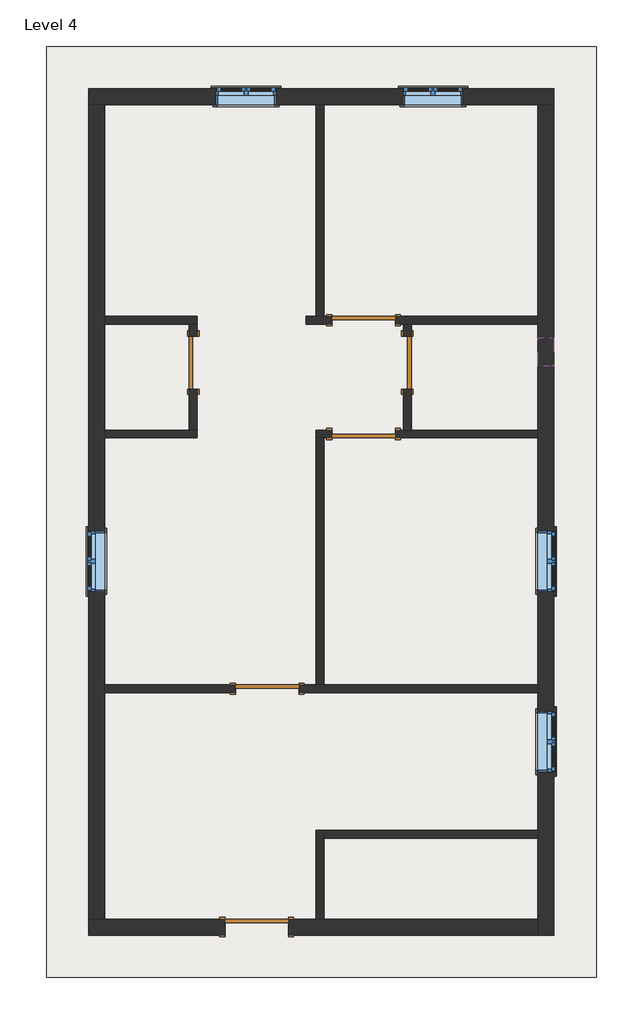
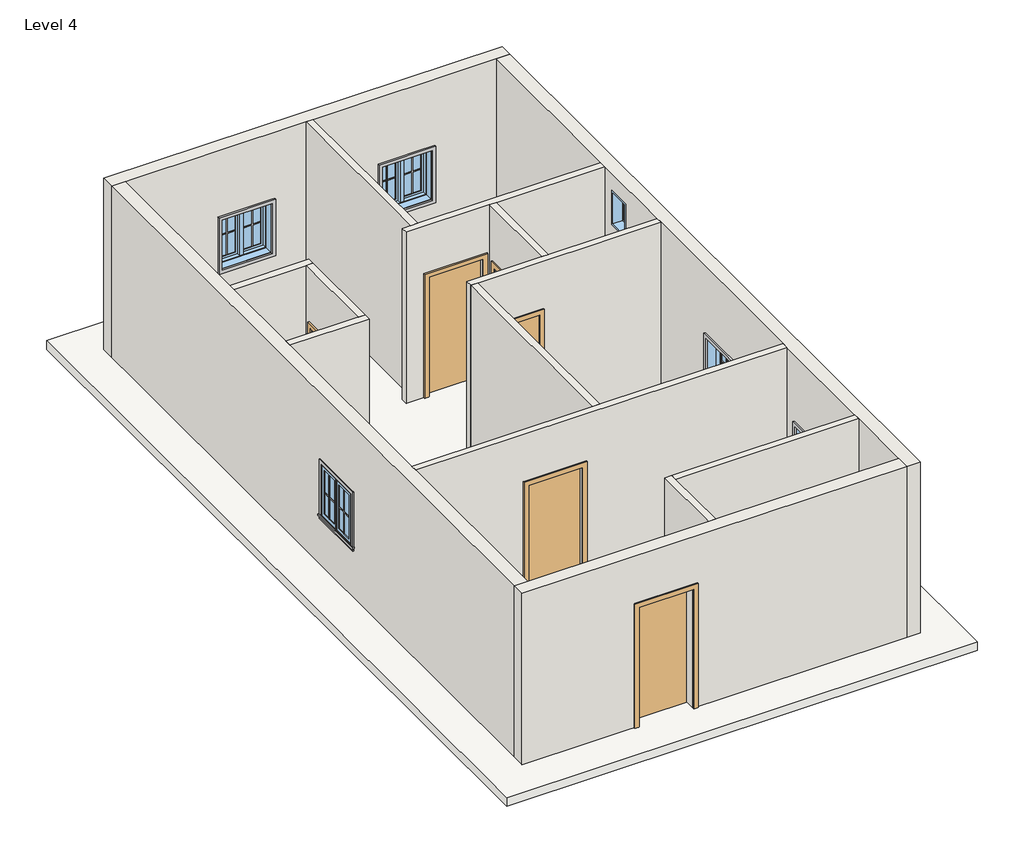
# One storey, incomplete: 20 proxies, 15 walls, 6 doors, 6 windows, 1 roof.
"""IFC4 building model written with IfcOpenShell, lengths in millimetres."""

from ifc_helpers import new_model, si_unit, frame, origin, place, context, project, spatial, polyline, outline, extrude, faceted_brep, transform, mapped, element, save
from components import muntin_pattern_2x2_muntin_pattern_2x2_b3fe6957, muntin_pattern_2x2_muntin_pattern_2x2_3e0ecaf2, trim_window_exterior_flat_with_sill_41619996, trim_window_interior_flat_picture_frame_51c85655, door_f2b275c1, door_d8f5dbb5, door_305aa2a5, door_e5f9f3c4, door_a90ba1ad, window_aa618e30, window_339605e1

model = new_model("IFC4")

# Units and contexts
model_context = context("Model", 3, world=origin())
ifc_project = project(units=[si_unit("LENGTHUNIT", "METRE", prefix="MILLI")], contexts=[model_context])

# Site, building, storey
site = spatial("IfcSite", under=ifc_project)
building = spatial("IfcBuilding", under=site)
storey = spatial("IfcBuildingStorey", under=building, Name="Level 4", Elevation=6400.8)

# Proxies
placement = place(None, origin())
muntin_pattern_2x2_muntin_pattern_2x2_shape = muntin_pattern_2x2_muntin_pattern_2x2_b3fe6957(model_context)
element("IfcBuildingElementProxy", 1, Name="Muntin Pattern_2x2 : Muntin Pattern_2x2", ObjectType="Muntin Pattern_2x2 : Muntin Pattern_2x2", at=placement, inside=storey, context=model_context, shape_type="MappedRepresentation", body=[
    mapped(muntin_pattern_2x2_muntin_pattern_2x2_shape, transform((-2560.703247, 6624.6685985, 7385.05), x_axis=(1.0, 0.0, 0.0), y_axis=(0.0, 1.0, 0.0), z_axis=(0.0, 0.0, 1.0))),
])
element("IfcBuildingElementProxy", 2, Name="Muntin Pattern_2x2 : Muntin Pattern_2x2", ObjectType="Muntin Pattern_2x2 : Muntin Pattern_2x2", at=placement, inside=storey, context=model_context, shape_type="MappedRepresentation", body=[
    mapped(muntin_pattern_2x2_muntin_pattern_2x2_shape, transform((134.871753, 6624.6685985, 7385.05), x_axis=(1.0, 0.0, 0.0), y_axis=(0.0, 1.0, 0.0), z_axis=(0.0, 0.0, 1.0))),
])
element("IfcBuildingElementProxy", 3, Name="Muntin Pattern_2x2 : Muntin Pattern_2x2", ObjectType="Muntin Pattern_2x2 : Muntin Pattern_2x2", at=placement, inside=storey, context=model_context, shape_type="MappedRepresentation", body=[
    mapped(muntin_pattern_2x2_muntin_pattern_2x2_shape, transform((2082.734253, 41.3060985, 7385.05), x_axis=(0.0, -1.0, 0.0), y_axis=(1.0, 0.0, 0.0), z_axis=(0.0, 0.0, 1.0))),
])
element("IfcBuildingElementProxy", 4, Name="Muntin Pattern_2x2 : Muntin Pattern_2x2", ObjectType="Muntin Pattern_2x2 : Muntin Pattern_2x2", at=placement, inside=storey, context=model_context, shape_type="MappedRepresentation", body=[
    mapped(muntin_pattern_2x2_muntin_pattern_2x2_shape, transform((-4603.815747, -387.3189015, 7385.05), x_axis=(0.0, 1.0, 0.0), y_axis=(-1.0, 0.0, 0.0), z_axis=(0.0, 0.0, 1.0))),
])
element("IfcBuildingElementProxy", 5, Name="Muntin Pattern_2x2 : Muntin Pattern_2x2", ObjectType="Muntin Pattern_2x2 : Muntin Pattern_2x2", at=placement, inside=storey, context=model_context, shape_type="MappedRepresentation", body=[
    mapped(muntin_pattern_2x2_muntin_pattern_2x2_shape, transform((2082.734253, -2555.8439015, 7385.05), x_axis=(0.0, -1.0, 0.0), y_axis=(1.0, 0.0, 0.0), z_axis=(0.0, 0.0, 1.0))),
])
muntin_pattern_2x2_muntin_pattern_2x2_2_shape = muntin_pattern_2x2_muntin_pattern_2x2_3e0ecaf2(model_context)
element("IfcBuildingElementProxy", 6, Name="Muntin Pattern_2x2 : Muntin Pattern_2x2", ObjectType="Muntin Pattern_2x2 : Muntin Pattern_2x2", at=placement, inside=storey, context=model_context, shape_type="MappedRepresentation", body=[
    mapped(muntin_pattern_2x2_muntin_pattern_2x2_2_shape, transform((-2132.078247, 6624.6685985, 7385.05), x_axis=(-1.0, 0.0, 0.0), y_axis=(0.0, -1.0, 0.0), z_axis=(0.0, 0.0, 1.0))),
])
element("IfcBuildingElementProxy", 7, Name="Muntin Pattern_2x2 : Muntin Pattern_2x2", ObjectType="Muntin Pattern_2x2 : Muntin Pattern_2x2", at=placement, inside=storey, context=model_context, shape_type="MappedRepresentation", body=[
    mapped(muntin_pattern_2x2_muntin_pattern_2x2_2_shape, transform((563.496753, 6624.6685985, 7385.05), x_axis=(-1.0, 0.0, 0.0), y_axis=(0.0, -1.0, 0.0), z_axis=(0.0, 0.0, 1.0))),
])
element("IfcBuildingElementProxy", 8, Name="Muntin Pattern_2x2 : Muntin Pattern_2x2", ObjectType="Muntin Pattern_2x2 : Muntin Pattern_2x2", at=placement, inside=storey, context=model_context, shape_type="MappedRepresentation", body=[
    mapped(muntin_pattern_2x2_muntin_pattern_2x2_2_shape, transform((2082.734253, -387.3189015, 7385.05), x_axis=(0.0, 1.0, 0.0), y_axis=(-1.0, 0.0, 0.0), z_axis=(0.0, 0.0, 1.0))),
])
element("IfcBuildingElementProxy", 9, Name="Muntin Pattern_2x2 : Muntin Pattern_2x2", ObjectType="Muntin Pattern_2x2 : Muntin Pattern_2x2", at=placement, inside=storey, context=model_context, shape_type="MappedRepresentation", body=[
    mapped(muntin_pattern_2x2_muntin_pattern_2x2_2_shape, transform((-4603.815747, 41.3060985, 7385.05), x_axis=(0.0, -1.0, 0.0), y_axis=(1.0, 0.0, 0.0), z_axis=(0.0, 0.0, 1.0))),
])
element("IfcBuildingElementProxy", 10, Name="Muntin Pattern_2x2 : Muntin Pattern_2x2", ObjectType="Muntin Pattern_2x2 : Muntin Pattern_2x2", at=placement, inside=storey, context=model_context, shape_type="MappedRepresentation", body=[
    mapped(muntin_pattern_2x2_muntin_pattern_2x2_2_shape, transform((2082.734253, -2984.4689015, 7385.05), x_axis=(0.0, 1.0, 0.0), y_axis=(-1.0, 0.0, 0.0), z_axis=(0.0, 0.0, 1.0))),
])
trim_window_exterior_flat_with_sill_shape = trim_window_exterior_flat_with_sill_41619996(model_context)
element("IfcBuildingElementProxy", 11, Name="Trim-Window-Exterior-Flat : with Sill", ObjectType="Trim-Window-Exterior-Flat : with Sill", at=placement, inside=storey, context=model_context, shape_type="MappedRepresentation", body=[
    mapped(trim_window_exterior_flat_with_sill_shape, transform((-2346.390747, 6634.1935985, 8229.6), x_axis=(-1.0, 0.0, 0.0), y_axis=(0.0, 0.0, 1.0), z_axis=(0.0, 1.0, 0.0))),
])
element("IfcBuildingElementProxy", 12, Name="Trim-Window-Exterior-Flat : with Sill", ObjectType="Trim-Window-Exterior-Flat : with Sill", at=placement, inside=storey, context=model_context, shape_type="MappedRepresentation", body=[
    mapped(trim_window_exterior_flat_with_sill_shape, transform((349.184253, 6634.1935985, 8229.6), x_axis=(-1.0, 0.0, 0.0), y_axis=(0.0, 0.0, 1.0), z_axis=(0.0, 1.0, 0.0))),
])
element("IfcBuildingElementProxy", 13, Name="Trim-Window-Exterior-Flat : with Sill", ObjectType="Trim-Window-Exterior-Flat : with Sill", at=placement, inside=storey, context=model_context, shape_type="MappedRepresentation", body=[
    mapped(trim_window_exterior_flat_with_sill_shape, transform((2092.259253, -173.0064015, 8229.6), x_axis=(0.0, 1.0, 0.0), y_axis=(0.0, 0.0, 1.0), z_axis=(1.0, 0.0, 0.0))),
])
element("IfcBuildingElementProxy", 14, Name="Trim-Window-Exterior-Flat : with Sill", ObjectType="Trim-Window-Exterior-Flat : with Sill", at=placement, inside=storey, context=model_context, shape_type="MappedRepresentation", body=[
    mapped(trim_window_exterior_flat_with_sill_shape, transform((-4613.340747, -173.0064015, 8229.6), x_axis=(0.0, -1.0, 0.0), y_axis=(0.0, 0.0, 1.0), z_axis=(-1.0, 0.0, 0.0))),
])
element("IfcBuildingElementProxy", 15, Name="Trim-Window-Exterior-Flat : with Sill", ObjectType="Trim-Window-Exterior-Flat : with Sill", at=placement, inside=storey, context=model_context, shape_type="MappedRepresentation", body=[
    mapped(trim_window_exterior_flat_with_sill_shape, transform((2092.259253, -2770.1564015, 8229.6), x_axis=(0.0, 1.0, 0.0), y_axis=(0.0, 0.0, 1.0), z_axis=(1.0, 0.0, 0.0))),
])
trim_window_interior_flat_picture_frame_shape = trim_window_interior_flat_picture_frame_51c85655(model_context)
element("IfcBuildingElementProxy", 16, Name="Trim-Window-Interior-Flat : Picture Frame", ObjectType="Trim-Window-Interior-Flat : Picture Frame", at=placement, inside=storey, context=model_context, shape_type="MappedRepresentation", body=[
    mapped(trim_window_interior_flat_picture_frame_shape, transform((-2346.390747, 6405.5935985, 8229.6), x_axis=(1.0, 0.0, 0.0), y_axis=(0.0, 0.0, 1.0), z_axis=(0.0, -1.0, 0.0))),
])
element("IfcBuildingElementProxy", 17, Name="Trim-Window-Interior-Flat : Picture Frame", ObjectType="Trim-Window-Interior-Flat : Picture Frame", at=placement, inside=storey, context=model_context, shape_type="MappedRepresentation", body=[
    mapped(trim_window_interior_flat_picture_frame_shape, transform((349.184253, 6405.5935985, 8229.6), x_axis=(1.0, 0.0, 0.0), y_axis=(0.0, 0.0, 1.0), z_axis=(0.0, -1.0, 0.0))),
])
element("IfcBuildingElementProxy", 18, Name="Trim-Window-Interior-Flat : Picture Frame", ObjectType="Trim-Window-Interior-Flat : Picture Frame", at=placement, inside=storey, context=model_context, shape_type="MappedRepresentation", body=[
    mapped(trim_window_interior_flat_picture_frame_shape, transform((1863.659253, -173.0064015, 8229.6), x_axis=(0.0, -1.0, 0.0), y_axis=(0.0, 0.0, 1.0), z_axis=(-1.0, 0.0, 0.0))),
])
element("IfcBuildingElementProxy", 19, Name="Trim-Window-Interior-Flat : Picture Frame", ObjectType="Trim-Window-Interior-Flat : Picture Frame", at=placement, inside=storey, context=model_context, shape_type="MappedRepresentation", body=[
    mapped(trim_window_interior_flat_picture_frame_shape, transform((-4384.740747, -173.0064015, 8229.6), x_axis=(0.0, 1.0, 0.0), y_axis=(0.0, 0.0, 1.0), z_axis=(1.0, 0.0, 0.0))),
])
element("IfcBuildingElementProxy", 20, Name="Trim-Window-Interior-Flat : Picture Frame", ObjectType="Trim-Window-Interior-Flat : Picture Frame", at=placement, inside=storey, context=model_context, shape_type="MappedRepresentation", body=[
    mapped(trim_window_interior_flat_picture_frame_shape, transform((1863.659253, -2770.1564015, 8229.6), x_axis=(0.0, -1.0, 0.0), y_axis=(0.0, 0.0, 1.0), z_axis=(-1.0, 0.0, 0.0))),
])

# Doors
door_shape = door_f2b275c1(model_context)
element("IfcDoor", 21, ObjectType="Single-Flush : 30\" x 80\"", at=placement, inside=storey, context=model_context, shape_type="MappedRepresentation", body=[
    mapped(door_shape, transform((-22.290747, 2690.8435985, 6400.8), x_axis=(0.0, 1.0, 0.0), y_axis=(-1.0, 0.0, 0.0), z_axis=(0.0, 0.0, 1.0))),
])
door_2_shape = door_d8f5dbb5(model_context)
element("IfcDoor", 22, ObjectType="Single-Flush : 30\" x 80\"", at=placement, inside=storey, context=model_context, shape_type="MappedRepresentation", body=[
    mapped(door_2_shape, transform((-3108.390747, 2690.8435985, 6400.8), x_axis=(0.0, 1.0, 0.0), y_axis=(-1.0, 0.0, 0.0), z_axis=(0.0, 0.0, 1.0))),
])
door_3_shape = door_305aa2a5(model_context)
element("IfcDoor", 23, ObjectType="Single-Flush : 36\" x 84\"", at=placement, inside=storey, context=model_context, shape_type="MappedRepresentation", body=[
    mapped(door_3_shape, transform((-650.940747, 3300.4435985, 6400.8), x_axis=(-1.0, 0.0, 0.0), y_axis=(0.0, -1.0, 0.0), z_axis=(0.0, 0.0, 1.0))),
])
door_4_shape = door_e5f9f3c4(model_context)
element("IfcDoor", 24, ObjectType="Single-Flush : 36\" x 84\"", at=placement, inside=storey, context=model_context, shape_type="MappedRepresentation", body=[
    mapped(door_4_shape, transform((-2041.590747, -2008.1564015, 6400.8), x_axis=(1.0, 0.0, 0.0), y_axis=(0.0, 1.0, 0.0), z_axis=(0.0, 0.0, 1.0))),
])
element("IfcDoor", 25, ObjectType="Single-Flush : 36\" x 84\"", at=placement, inside=storey, context=model_context, shape_type="MappedRepresentation", body=[
    mapped(door_4_shape, transform((-650.940747, 1662.1435985, 6400.8), x_axis=(-1.0, 0.0, 0.0), y_axis=(0.0, -1.0, 0.0), z_axis=(0.0, 0.0, 1.0))),
])
door_5_shape = door_a90ba1ad(model_context)
element("IfcDoor", 26, ObjectType="Single-Flush : 36\" x 84\"", at=placement, inside=storey, context=model_context, shape_type="MappedRepresentation", body=[
    mapped(door_5_shape, transform((-2193.990747, -5443.5064015, 6400.8), x_axis=(-1.0, 0.0, 0.0), y_axis=(0.0, -1.0, 0.0), z_axis=(0.0, 0.0, 1.0))),
])

# Roof
element("IfcRoof", 27, ObjectType="Generic - 12\"", at=placement, inside=storey, context=model_context, shape_type="SweptSolid", body=[
    extrude(outline(polyline([(-5222.940747, 7243.7935985), (2701.859253, 7243.7935985), (2701.859253, -6167.4064015), (-5222.940747, -6167.4064015), (-5222.940747, 7243.7935985)])), frame((0.0, 0.0, 6248.4), z_axis=(0.0, 0.0, 1.0), x_axis=(1.0, 0.0, 0.0)), (0.0, 0.0, 1.0), 152.4),
])

# Walls
element("IfcWall", 28, ObjectType="WALL4.5\"", at=placement, inside=storey, context=model_context, shape_type="Brep", body=[
    faceted_brep([(-4384.740747, 3243.2935985, 6400.8), (-3165.540747, 3243.2935985, 6400.8), (-3051.240747, 3243.2935985, 6400.8), (-3051.240747, 3243.2935985, 9448.8), (-3165.540747, 3243.2935985, 9448.8), (-4384.740747, 3243.2935985, 9448.8), (-4384.740747, 3357.5935985, 6400.8), (-4384.740747, 3357.5935985, 9448.8), (-3051.240747, 3357.5935985, 9448.8), (-3051.240747, 3357.5935985, 6400.8)], [[[0, 1, 2, 3, 4, 5]], [[6, 7, 8, 9]], [[2, 1, 0, 6, 9]], [[0, 5, 7, 6]], [[3, 2, 9, 8]], [[5, 4, 3, 8, 7]]]),
])
element("IfcWall", 29, ObjectType="WALL4.5\"", at=placement, inside=storey, context=model_context, shape_type="Brep", body=[
    faceted_brep([(-4384.740747, 1604.9935985, 6400.8), (-3051.240747, 1604.9935985, 6400.8), (-3051.240747, 1604.9935985, 9448.8), (-4384.740747, 1604.9935985, 9448.8), (-4384.740747, 1719.2935985, 6400.8), (-4384.740747, 1719.2935985, 9448.8), (-3165.540747, 1719.2935985, 9448.8), (-3051.240747, 1719.2935985, 9448.8), (-3051.240747, 1719.2935985, 6400.8), (-3165.540747, 1719.2935985, 6400.8)], [[[0, 1, 2, 3]], [[4, 5, 6, 7, 8, 9]], [[1, 0, 4, 9, 8]], [[0, 3, 5, 4]], [[2, 1, 8, 7]], [[3, 2, 7, 6, 5]]]),
])
element("IfcWall", 30, ObjectType="WALL4.5\"", at=placement, inside=storey, context=model_context, shape_type="SweptSolid", body=[
    extrude(outline(polyline([(3243.2935985, 6400.8), (3071.8435985, 6400.8), (3071.8435985, 8432.8), (2309.8435985, 8432.8), (2309.8435985, 6400.8), (1719.2935985, 6400.8), (1719.2935985, 9448.8), (3243.2935985, 9448.8), (3243.2935985, 6400.8)])), frame((-3165.540747, 0.0, 0.0), z_axis=(1.0, 0.0, 0.0), x_axis=(0.0, 1.0, 0.0)), (0.0, 0.0, 1.0), 114.3),
])
element("IfcWall", 31, ObjectType="WALL4.5\"", at=placement, inside=storey, context=model_context, shape_type="SweptSolid", body=[
    extrude(outline(polyline([(-1336.740747, 3357.5935985), (-1336.740747, 6405.5935985), (-1222.440747, 6405.5935985), (-1222.440747, 3357.5935985), (-1336.740747, 3357.5935985)])), frame((0.0, 0.0, 6400.8), z_axis=(0.0, 0.0, 1.0), x_axis=(1.0, 0.0, 0.0)), (0.0, 0.0, 1.0), 3048.0),
])
element("IfcWall", 32, ObjectType="WALL4.5\"", at=placement, inside=storey, context=model_context, shape_type="Brep", body=[
    faceted_brep([(-1481.7019184, 3243.2935985, 6400.8), (-1108.140747, 3243.2935985, 6400.8), (-1108.140747, 3243.2935985, 8534.4), (-193.740747, 3243.2935985, 8534.4), (-193.740747, 3243.2935985, 6400.8), (-79.440747, 3243.2935985, 6400.8), (34.859253, 3243.2935985, 6400.8), (1863.659253, 3243.2935985, 6400.8), (1863.659253, 3243.2935985, 9448.8), (34.859253, 3243.2935985, 9448.8), (-79.440747, 3243.2935985, 9448.8), (-1481.7019184, 3243.2935985, 9448.8), (-1108.140747, 3357.5935985, 8534.4), (-1108.140747, 3357.5935985, 6400.8), (-1222.440747, 3357.5935985, 6400.8), (-1336.740747, 3357.5935985, 6400.8), (-1481.7019184, 3357.5935985, 6400.8), (-1481.7019184, 3357.5935985, 9448.8), (-1336.740747, 3357.5935985, 9448.8), (-1222.440747, 3357.5935985, 9448.8), (1863.659253, 3357.5935985, 9448.8), (1863.659253, 3357.5935985, 6400.8), (-193.740747, 3357.5935985, 6400.8), (-193.740747, 3357.5935985, 8534.4)], [[[0, 1, 2, 3, 4, 5, 6, 7, 8, 9, 10, 11]], [[12, 13, 14, 15, 16, 17, 18, 19, 20, 21, 22, 23]], [[22, 21, 7, 6, 5, 4]], [[16, 15, 14, 13, 1, 0]], [[0, 11, 17, 16]], [[8, 7, 21, 20]], [[2, 1, 13, 12]], [[3, 2, 12, 23]], [[4, 3, 23, 22]], [[11, 10, 9, 8, 20, 19, 18, 17]]]),
])
element("IfcWall", 33, ObjectType="WALL4.5\"", at=placement, inside=storey, context=model_context, shape_type="SweptSolid", body=[
    extrude(outline(polyline([(3243.2935985, 6400.8), (3071.8435985, 6400.8), (3071.8435985, 8432.8), (2309.8435985, 8432.8), (2309.8435985, 6400.8), (1719.2935985, 6400.8), (1719.2935985, 9448.8), (3243.2935985, 9448.8), (3243.2935985, 6400.8)])), frame((-79.440747, 0.0, 0.0), z_axis=(1.0, 0.0, 0.0), x_axis=(0.0, 1.0, 0.0)), (0.0, 0.0, 1.0), 114.3),
])
element("IfcWall", 34, ObjectType="WALL4.5\"", at=placement, inside=storey, context=model_context, shape_type="Brep", body=[
    faceted_brep([(-1108.140747, 1719.2935985, 8534.4), (-1108.140747, 1719.2935985, 6400.8), (-1336.740747, 1719.2935985, 6400.8), (-1336.740747, 1719.2935985, 9448.8), (-79.440747, 1719.2935985, 9448.8), (34.859253, 1719.2935985, 9448.8), (1863.659253, 1719.2935985, 9448.8), (1863.659253, 1719.2935985, 6400.8), (34.859253, 1719.2935985, 6400.8), (-79.440747, 1719.2935985, 6400.8), (-193.740747, 1719.2935985, 6400.8), (-193.740747, 1719.2935985, 8534.4), (-1336.740747, 1604.9935985, 6400.8), (-1222.440747, 1604.9935985, 6400.8), (-1108.140747, 1604.9935985, 6400.8), (-1108.140747, 1604.9935985, 8534.4), (-193.740747, 1604.9935985, 8534.4), (-193.740747, 1604.9935985, 6400.8), (1863.659253, 1604.9935985, 6400.8), (1863.659253, 1604.9935985, 9448.8), (-1222.440747, 1604.9935985, 9448.8), (-1336.740747, 1604.9935985, 9448.8)], [[[0, 1, 2, 3, 4, 5, 6, 7, 8, 9, 10, 11]], [[12, 13, 14, 15, 16, 17, 18, 19, 20, 21]], [[2, 1, 14, 13, 12]], [[10, 9, 8, 7, 18, 17]], [[7, 6, 19, 18]], [[3, 2, 12, 21]], [[15, 14, 1, 0]], [[16, 15, 0, 11]], [[17, 16, 11, 10]], [[6, 5, 4, 3, 21, 20, 19]]]),
])
element("IfcWall", 35, ObjectType="WALL4.5\"", at=placement, inside=storey, context=model_context, shape_type="SweptSolid", body=[
    extrude(outline(polyline([(-1336.740747, -1951.0064015), (-1336.740747, 1604.9935985), (-1222.440747, 1604.9935985), (-1222.440747, -1951.0064015), (-1336.740747, -1951.0064015)])), frame((0.0, 0.0, 6400.8), z_axis=(0.0, 0.0, 1.0), x_axis=(1.0, 0.0, 0.0)), (0.0, 0.0, 1.0), 3048.0),
])
element("IfcWall", 36, ObjectType="WALL4.5\"", at=placement, inside=storey, context=model_context, shape_type="Brep", body=[
    faceted_brep([(-1584.390747, -2065.3064015, 8534.4), (-1584.390747, -2065.3064015, 6400.8), (1863.659253, -2065.3064015, 6400.8), (1863.659253, -2065.3064015, 9448.8), (-4384.740747, -2065.3064015, 9448.8), (-4384.740747, -2065.3064015, 6400.8), (-2498.790747, -2065.3064015, 6400.8), (-2498.790747, -2065.3064015, 8534.4), (1863.659253, -1951.0064015, 6400.8), (-1222.440747, -1951.0064015, 6400.8), (-1336.740747, -1951.0064015, 6400.8), (-1584.390747, -1951.0064015, 6400.8), (-1584.390747, -1951.0064015, 8534.4), (-2498.790747, -1951.0064015, 8534.4), (-2498.790747, -1951.0064015, 6400.8), (-4384.740747, -1951.0064015, 6400.8), (-4384.740747, -1951.0064015, 9448.8), (-1336.740747, -1951.0064015, 9448.8), (-1222.440747, -1951.0064015, 9448.8), (1863.659253, -1951.0064015, 9448.8)], [[[0, 1, 2, 3, 4, 5, 6, 7]], [[8, 9, 10, 11, 12, 13, 14, 15, 16, 17, 18, 19]], [[6, 5, 15, 14]], [[2, 1, 11, 10, 9, 8]], [[3, 2, 8, 19]], [[5, 4, 16, 15]], [[12, 11, 1, 0]], [[13, 12, 0, 7]], [[14, 13, 7, 6]], [[4, 3, 19, 18, 17, 16]]]),
])
element("IfcWall", 37, ObjectType="WALL4.5\"", at=placement, inside=storey, context=model_context, shape_type="Brep", body=[
    faceted_brep([(-1222.440747, -5329.2064015, 6400.8), (-1222.440747, -4160.8064015, 6400.8), (-1222.440747, -4046.5064015, 6400.8), (-1222.440747, -4046.5064015, 9448.8), (-1222.440747, -4160.8064015, 9448.8), (-1222.440747, -5329.2064015, 9448.8), (-1336.740747, -5329.2064015, 6400.8), (-1336.740747, -5329.2064015, 9448.8), (-1336.740747, -4046.5064015, 9448.8), (-1336.740747, -4046.5064015, 6400.8)], [[[0, 1, 2, 3, 4, 5]], [[6, 7, 8, 9]], [[2, 1, 0, 6, 9]], [[0, 5, 7, 6]], [[3, 2, 9, 8]], [[5, 4, 3, 8, 7]]]),
])
element("IfcWall", 38, ObjectType="WALL4.5\"", at=placement, inside=storey, context=model_context, shape_type="SweptSolid", body=[
    extrude(outline(polyline([(1863.659253, -4160.8064015), (-1222.440747, -4160.8064015), (-1222.440747, -4046.5064015), (1863.659253, -4046.5064015), (1863.659253, -4160.8064015)])), frame((0.0, 0.0, 6400.8), z_axis=(0.0, 0.0, 1.0), x_axis=(1.0, 0.0, 0.0)), (0.0, 0.0, 1.0), 3048.0),
])
element("IfcWall", 39, ObjectType="WALL9\"", at=placement, inside=storey, context=model_context, shape_type="Brep", body=[
    faceted_brep([(-4613.340747, 6405.5935985, 6400.8), (-4384.740747, 6405.5935985, 6400.8), (-1336.740747, 6405.5935985, 6400.8), (-1222.440747, 6405.5935985, 6400.8), (1863.659253, 6405.5935985, 6400.8), (2092.259253, 6405.5935985, 6400.8), (2092.259253, 6405.5935985, 9448.8), (1863.659253, 6405.5935985, 9448.8), (-1222.440747, 6405.5935985, 9448.8), (-1336.740747, 6405.5935985, 9448.8), (-4384.740747, 6405.5935985, 9448.8), (-4613.340747, 6405.5935985, 9448.8), (-1914.590747, 6405.5935985, 8229.6), (-1914.590747, 6405.5935985, 7315.2), (-2778.190747, 6405.5935985, 7315.2), (-2778.190747, 6405.5935985, 8229.6), (780.984253, 6405.5935985, 8229.6), (780.984253, 6405.5935985, 7315.2), (-82.615747, 6405.5935985, 7315.2), (-82.615747, 6405.5935985, 8229.6), (-4613.340747, 6634.1935985, 6400.8), (-4613.340747, 6634.1935985, 9448.8), (2092.259253, 6634.1935985, 9448.8), (2092.259253, 6634.1935985, 6400.8), (-1914.590747, 6634.1935985, 8229.6), (-2778.190747, 6634.1935985, 8229.6), (-2778.190747, 6634.1935985, 7315.2), (-1914.590747, 6634.1935985, 7315.2), (780.984253, 6634.1935985, 8229.6), (-82.615747, 6634.1935985, 8229.6), (-82.615747, 6634.1935985, 7315.2), (780.984253, 6634.1935985, 7315.2)], [[[0, 1, 2, 3, 4, 5, 6, 7, 8, 9, 10, 11], [12, 13, 14, 15], [16, 17, 18, 19]], [[20, 21, 22, 23], [24, 25, 26, 27], [28, 29, 30, 31]], [[5, 4, 3, 2, 1, 0, 20, 23]], [[6, 5, 23, 22]], [[0, 11, 21, 20]], [[13, 12, 24, 27]], [[14, 13, 27, 26]], [[15, 14, 26, 25]], [[12, 15, 25, 24]], [[17, 16, 28, 31]], [[18, 17, 31, 30]], [[19, 18, 30, 29]], [[16, 19, 29, 28]], [[11, 10, 9, 8, 7, 6, 22, 21]]]),
])
element("IfcWall", 40, ObjectType="WALL9\"", at=placement, inside=storey, context=model_context, shape_type="Brep", body=[
    faceted_brep([(1863.659253, 6405.5935985, 6400.8), (1863.659253, 3357.5935985, 6400.8), (1863.659253, 3243.2935985, 6400.8), (1863.659253, 1719.2935985, 6400.8), (1863.659253, 1604.9935985, 6400.8), (1863.659253, -1951.0064015, 6400.8), (1863.659253, -2065.3064015, 6400.8), (1863.659253, -4046.5064015, 6400.8), (1863.659253, -4160.8064015, 6400.8), (1863.659253, -5329.2064015, 6400.8), (1863.659253, -5557.8064015, 6400.8), (1863.659253, -5557.8064015, 9448.8), (1863.659253, -5329.2064015, 9448.8), (1863.659253, -4160.8064015, 9448.8), (1863.659253, -4046.5064015, 9448.8), (1863.659253, -2065.3064015, 9448.8), (1863.659253, -1951.0064015, 9448.8), (1863.659253, 1604.9935985, 9448.8), (1863.659253, 1719.2935985, 9448.8), (1863.659253, 3243.2935985, 9448.8), (1863.659253, 3357.5935985, 9448.8), (1863.659253, 6405.5935985, 9448.8), (1863.659253, 2640.0435985, 9144.0), (1863.659253, 2640.0435985, 8534.4), (1863.659253, 3046.4435985, 8534.4), (1863.659253, 3046.4435985, 9144.0), (1863.659253, -604.8064015, 8229.6), (1863.659253, -604.8064015, 7315.2), (1863.659253, 258.7935985, 7315.2), (1863.659253, 258.7935985, 8229.6), (1863.659253, -3201.9564015, 8229.6), (1863.659253, -3201.9564015, 7315.2), (1863.659253, -2338.3564015, 7315.2), (1863.659253, -2338.3564015, 8229.6), (2092.259253, 6405.5935985, 6400.8), (2092.259253, 6405.5935985, 9448.8), (2092.259253, -5557.8064015, 9448.8), (2092.259253, -5557.8064015, 6400.8), (2092.259253, 2640.0435985, 9144.0), (2092.259253, 3046.4435985, 9144.0), (2092.259253, 3046.4435985, 8534.4), (2092.259253, 2640.0435985, 8534.4), (2092.259253, -604.8064015, 8229.6), (2092.259253, 258.7935985, 8229.6), (2092.259253, 258.7935985, 7315.2), (2092.259253, -604.8064015, 7315.2), (2092.259253, -3201.9564015, 8229.6), (2092.259253, -2338.3564015, 8229.6), (2092.259253, -2338.3564015, 7315.2), (2092.259253, -3201.9564015, 7315.2)], [[[0, 1, 2, 3, 4, 5, 6, 7, 8, 9, 10, 11, 12, 13, 14, 15, 16, 17, 18, 19, 20, 21], [22, 23, 24, 25], [26, 27, 28, 29], [30, 31, 32, 33]], [[34, 35, 36, 37], [38, 39, 40, 41], [42, 43, 44, 45], [46, 47, 48, 49]], [[10, 9, 8, 7, 6, 5, 4, 3, 2, 1, 0, 34, 37]], [[0, 21, 35, 34]], [[11, 10, 37, 36]], [[23, 22, 38, 41]], [[24, 23, 41, 40]], [[25, 24, 40, 39]], [[22, 25, 39, 38]], [[27, 26, 42, 45]], [[28, 27, 45, 44]], [[29, 28, 44, 43]], [[26, 29, 43, 42]], [[31, 30, 46, 49]], [[32, 31, 49, 48]], [[33, 32, 48, 47]], [[30, 33, 47, 46]], [[21, 20, 19, 18, 17, 16, 15, 14, 13, 12, 11, 36, 35]]]),
])
element("IfcWall", 41, ObjectType="WALL9\"", at=placement, inside=storey, context=model_context, shape_type="Brep", body=[
    faceted_brep([(-2651.190747, -5329.2064015, 8534.4), (-2651.190747, -5329.2064015, 6400.8), (-4384.740747, -5329.2064015, 6400.8), (-4613.340747, -5329.2064015, 6400.8), (-4613.340747, -5329.2064015, 9448.8), (-4384.740747, -5329.2064015, 9448.8), (-1336.740747, -5329.2064015, 9448.8), (-1222.440747, -5329.2064015, 9448.8), (1863.659253, -5329.2064015, 9448.8), (1863.659253, -5329.2064015, 6400.8), (-1222.440747, -5329.2064015, 6400.8), (-1336.740747, -5329.2064015, 6400.8), (-1736.790747, -5329.2064015, 6400.8), (-1736.790747, -5329.2064015, 8534.4), (-4613.340747, -5557.8064015, 6400.8), (-2651.190747, -5557.8064015, 6400.8), (-2651.190747, -5557.8064015, 8534.4), (-1736.790747, -5557.8064015, 8534.4), (-1736.790747, -5557.8064015, 6400.8), (1863.659253, -5557.8064015, 6400.8), (1863.659253, -5557.8064015, 9448.8), (-4613.340747, -5557.8064015, 9448.8)], [[[0, 1, 2, 3, 4, 5, 6, 7, 8, 9, 10, 11, 12, 13]], [[14, 15, 16, 17, 18, 19, 20, 21]], [[3, 2, 1, 15, 14]], [[12, 11, 10, 9, 19, 18]], [[9, 8, 20, 19]], [[4, 3, 14, 21]], [[16, 15, 1, 0]], [[17, 16, 0, 13]], [[18, 17, 13, 12]], [[8, 7, 6, 5, 4, 21, 20]]]),
])
element("IfcWall", 42, ObjectType="WALL9\"", at=placement, inside=storey, context=model_context, shape_type="Brep", body=[
    faceted_brep([(-4384.740747, -5329.2064015, 6400.8), (-4384.740747, -2065.3064015, 6400.8), (-4384.740747, -1951.0064015, 6400.8), (-4384.740747, 1604.9935985, 6400.8), (-4384.740747, 1719.2935985, 6400.8), (-4384.740747, 3243.2935985, 6400.8), (-4384.740747, 3357.5935985, 6400.8), (-4384.740747, 6405.5935985, 6400.8), (-4384.740747, 6405.5935985, 9448.8), (-4384.740747, 3357.5935985, 9448.8), (-4384.740747, 3243.2935985, 9448.8), (-4384.740747, 1719.2935985, 9448.8), (-4384.740747, 1604.9935985, 9448.8), (-4384.740747, -1951.0064015, 9448.8), (-4384.740747, -2065.3064015, 9448.8), (-4384.740747, -5329.2064015, 9448.8), (-4384.740747, 258.7935985, 8229.6), (-4384.740747, 258.7935985, 7315.2), (-4384.740747, -604.8064015, 7315.2), (-4384.740747, -604.8064015, 8229.6), (-4613.340747, -5329.2064015, 6400.8), (-4613.340747, -5329.2064015, 9448.8), (-4613.340747, 6405.5935985, 9448.8), (-4613.340747, 6405.5935985, 6400.8), (-4613.340747, 258.7935985, 8229.6), (-4613.340747, -604.8064015, 8229.6), (-4613.340747, -604.8064015, 7315.2), (-4613.340747, 258.7935985, 7315.2)], [[[0, 1, 2, 3, 4, 5, 6, 7, 8, 9, 10, 11, 12, 13, 14, 15], [16, 17, 18, 19]], [[20, 21, 22, 23], [24, 25, 26, 27]], [[7, 6, 5, 4, 3, 2, 1, 0, 20, 23]], [[8, 7, 23, 22]], [[0, 15, 21, 20]], [[17, 16, 24, 27]], [[18, 17, 27, 26]], [[19, 18, 26, 25]], [[16, 19, 25, 24]], [[15, 14, 13, 12, 11, 10, 9, 8, 22, 21]]]),
])

# Windows
window_shape = window_aa618e30(model_context)
element("IfcWindow", 43, ObjectType="Fixed : 16\" x 24\"", at=placement, inside=storey, context=model_context, shape_type="MappedRepresentation", body=[
    mapped(window_shape, transform((1977.959253, 2805.1435985, 7620.0), x_axis=(0.0, -1.0, 0.0), y_axis=(1.0, 0.0, 0.0), z_axis=(0.0, 0.0, 1.0))),
])
window_2_shape = window_339605e1(model_context)
element("IfcWindow", 44, ObjectType="Window-Casement-Double : 34\" x 36\"", at=placement, inside=storey, context=model_context, shape_type="MappedRepresentation", body=[
    mapped(window_2_shape, transform((-2346.390747, 6519.8935985, 6400.8), x_axis=(1.0, 0.0, 0.0), y_axis=(0.0, 1.0, 0.0), z_axis=(0.0, 0.0, 1.0))),
])
element("IfcWindow", 45, ObjectType="Window-Casement-Double : 34\" x 36\"", at=placement, inside=storey, context=model_context, shape_type="MappedRepresentation", body=[
    mapped(window_2_shape, transform((349.184253, 6519.8935985, 6400.8), x_axis=(1.0, 0.0, 0.0), y_axis=(0.0, 1.0, 0.0), z_axis=(0.0, 0.0, 1.0))),
])
element("IfcWindow", 46, ObjectType="Window-Casement-Double : 34\" x 36\"", at=placement, inside=storey, context=model_context, shape_type="MappedRepresentation", body=[
    mapped(window_2_shape, transform((1977.959253, -173.0064015, 6400.8), x_axis=(0.0, -1.0, 0.0), y_axis=(1.0, 0.0, 0.0), z_axis=(0.0, 0.0, 1.0))),
])
element("IfcWindow", 47, ObjectType="Window-Casement-Double : 34\" x 36\"", at=placement, inside=storey, context=model_context, shape_type="MappedRepresentation", body=[
    mapped(window_2_shape, transform((-4499.040747, -173.0064015, 6400.8), x_axis=(0.0, 1.0, 0.0), y_axis=(-1.0, 0.0, 0.0), z_axis=(0.0, 0.0, 1.0))),
])
element("IfcWindow", 48, ObjectType="Window-Casement-Double : 34\" x 36\"", at=placement, inside=storey, context=model_context, shape_type="MappedRepresentation", body=[
    mapped(window_2_shape, transform((1977.959253, -2770.1564015, 6400.8), x_axis=(0.0, -1.0, 0.0), y_axis=(1.0, 0.0, 0.0), z_axis=(0.0, 0.0, 1.0))),
])

save(model, "model.ifc")

# Revit data of these elements
# Type "Muntin Pattern_2x2 : Muntin Pattern_2x2"
#   Width [instance default] = 4' - 0"
#   Thickness = 0' - 0 1/2"
#   Height [instance default] = 4' - 0"
#   Distance = 0' - 0 3/4"
#   Interior Material [instance default] = none
#   Exterior Material [instance default] = none
#   Default Elevation = 0
# Type "Trim-Window-Exterior-Flat : with Sill"
#   Trim Width = 0' - 2 1/4"
#   Trim Thickness_Picture Frame = 0' - 1 1/4"
#   Trim Thickness_with Sill = 0' - 0 3/4"
#   Sill Thickness = 0' - 1 1/4"
#   Opening Width [instance default] = 2' - 0"
#   Opening Height [instance default] = 3' - 0"
#   Default Elevation = 4' - 0"
#   Sill = yes
#   Picture Frame = no
#   Trim Material [instance default] = none
# Type "Trim-Window-Interior-Flat : Picture Frame"
#   Trim Thickness_Picture Frame = 0' - 1 1/4"
#   Trim Width = 0' - 2 1/4"
#   Trim Thickness_with Sill = 0' - 0 3/4"
#   Sill Thickness = 0' - 1 1/4"
#   Opening Width [instance default] = 2' - 0"
#   Opening Height [instance default] = 3' - 0"
#   Default Elevation = 4' - 0"
#   Sill = no
#   Picture Frame = yes
#   Trim Material [instance default] = none
# Type "Single-Flush : 30\" x 80\""
#   Type Mark = "5"
#   Construction Type Id = "MDOOR"
#   Assembly Code = "C1020"
#   Analytic Construction = "Metal"
#   Thickness = 0' - 2"
#   Heat Transfer Coefficient (U) = 0.651978 BTU/(h·ft²·°F)
#   Height = 6' - 8"
#   Trim Projection Ext = 0' - 1"
#   Trim Projection Int = 0' - 1"
#   Trim Width = 0' - 3"
#   Width = 2' - 6"
#   Define Thermal Properties by = 1
#   Define Thermal Properties by = 1
#   Door Material = Door - Panel
#   Frame Material = Door - Frame
#   Visual Light Transmittance = 0
#   Solar Heat Gain Coefficient = 0
#   Function = (empty or 0)
#   Wall Closure = (empty or 0)
# Type "Single-Flush : 36\" x 84\""
#   Type Mark = "1"
#   Construction Type Id = "MDOOR"
#   Assembly Code = "C1020"
#   Analytic Construction = "Metal"
#   Thickness = 0' - 2"
#   Heat Transfer Coefficient (U) = 0.651978 BTU/(h·ft²·°F)
#   Height = 7' - 0"
#   Trim Projection Ext = 0' - 1"
#   Trim Projection Int = 0' - 1"
#   Trim Width = 0' - 3"
#   Width = 3' - 0"
#   Define Thermal Properties by = 1
#   Define Thermal Properties by = 1
#   Door Material = Door - Panel
#   Frame Material = Door - Frame
#   Visual Light Transmittance = 0
#   Solar Heat Gain Coefficient = 0
#   Function = (empty or 0)
#   Wall Closure = (empty or 0)
# Type "Generic - 12\""
#   Assembly Code = "B1020"
#   Layers, outside or top first: 0' - 6" no material (function 1)
# Type "WALL4.5\""
#   Assembly Code = "B2010"
#   Layers, outside or top first: 0' - 4 1/2" no material (function 1)
# Type "WALL9\""
#   Assembly Code = "B2010"
#   Layers, outside or top first: 0' - 9" no material (function 1)
# Type "Fixed : 16\" x 24\""
#   Type Mark = "4"
#   Construction Type Id = "GSP4R"
#   Assembly Code = "B2020100"
#   Analytic Construction = "1/8 in Pilkington single glazing"
#   Visual Light Transmittance = 0.9
#   Solar Heat Gain Coefficient = 0.78
#   Heat Transfer Coefficient (U) = 0.6496 BTU/(h·ft²·°F)
#   Height = 2' - 0"
#   Default Sill Height = 3' - 0"
#   Width = 1' - 4"
#   Window Inset = 0' - 0 3/4"
#   Define Thermal Properties by = 1
#   Define Thermal Properties by = 1
#   Glass Pane Material = Glass
#   Sash Material = Sash
#   Wall Closure = (empty or 0)
# Type "Window-Casement-Double : 34\" x 36\""
#   Type Mark = "14"
#   Fire Rating = "0.5h"
#   Assembly Code = "B2020100"
#   Analytic Construction = "Double glazing - domestic"
#   Frame Extension [instance default] = 0' - 0 1/4"
#   Window Inset [instance default] = 0' - 0"
#   Wall Thickness [instance default] = 0' - 6"
#   Interior Wall Closure [instance default] = 0' - 2 1/4"
#   Half Width = 1' - 5"
#   Visual Light Transmittance = 0.81
#   Thermal Resistance (R) = 1.8146 (h·ft²·°F)/BTU
#   Solar Heat Gain Coefficient = 0.76
#   Rough Width = 2' - 10 1/2"
#   Rough Height = 3' - 0 1/2"
#   Height = 3' - 0"
#   Heat Transfer Coefficient (U) = 0.5511 BTU/(h·ft²·°F)
#   Exterior Wall Closure [instance default] = 0' - 1 1/4"
#   Extension Jamb [instance default] = 0' - 2 1/4"
#   Default Sill Height = 3' - 0"
#   Width = 2' - 10"
#   Define Thermal Properties by = 0
#   Muntin Visibility = yes
#   Interior Trim Visibility [instance default] = yes
#   Exterior Trim Visibility [instance default] = yes
#   Extension Jamb Visibility [instance default] = yes
#   Interior Trim Material = Wood - Stained
#   Muntin Pattern = Muntin Pattern_2x2 : Muntin Pattern_2x2
#   Interior Trim = Trim-Window-Interior-Flat : Picture Frame
#   Interior Frame Material = Wood - Stained
#   Glass Panel Material = Glass
#   Exterior Trim Material = Clad - White
#   Exterior Trim = Trim-Window-Exterior-Flat : with Sill
#   Exterior Frame Material = Clad - White
#   Wall Closure = (empty or 0)
# Elements 1, 2, 3, 4, 5, 6, 7, 8, 9, 10 (IfcBuildingElementProxy, "Muntin Pattern_2x2 : Muntin Pattern_2x2")
#   Width = 0' - 11 5/8"
#   Height = 2' - 6 1/2"
#   Interior Material = Wood - Stained
#   Exterior Material = Clad - White
#   Phase Created = New Construction
#   Materials on its faces: "Clad - White", "Wood - Stained"
# Elements 11, 12, 13, 14, 15 (IfcBuildingElementProxy, "Trim-Window-Exterior-Flat : with Sill")
#   Opening Width = 2' - 10"
#   Opening Height = 3' - 0"
#   Trim Material = Clad - White
#   Phase Created = New Construction
#   Materials on its faces: "Clad - White"
# Elements 16, 17, 18, 19, 20 (IfcBuildingElementProxy, "Trim-Window-Interior-Flat : Picture Frame")
#   Opening Width = 2' - 10"
#   Opening Height = 3' - 0"
#   Trim Material = Wood - Stained
#   Phase Created = New Construction
#   Materials on its faces: "Wood - Stained"
# Elements 21, 22 (IfcDoor, "Single-Flush : 30\" x 80\"")
#   Phase Created = New Construction
#   Materials on its faces: "Door - Frame", "Door - Panel"
# Elements 23, 24, 25, 26 (IfcDoor, "Single-Flush : 36\" x 84\"")
#   Phase Created = New Construction
#   Materials on its faces: "Door - Frame", "Door - Panel"
# Element 27 (IfcRoof, "Generic - 12\"")
#   built-in parameter 1001705 = 21 (stored number, unit not read)
#   built-in parameter 1001701 = -0.5 (stored number, unit not read)
#   built-in parameter 1001710 = 33615
#   Phase Created = New Construction
#   Materials on its faces: "Default Roof"
# Elements 28, 29, 30, 31, 32, 33, 34, 35, 36, 37, 38 (IfcWall, "WALL4.5\"")
#   Top Offset = 0' - 0"
#   Base Offset = 0' - 0"
#   Unconnected Height = 10' - 0"
#   wall height = 10' - 0"
#   Phase Created = New Construction
#   Base Constraint = Level 4
#   Materials on its faces: "Default Wall"
# Elements 39, 40, 41, 42 (IfcWall, "WALL9\"")
#   Top Offset = 0' - 0"
#   Base Offset = 0' - 0"
#   Unconnected Height = 10' - 0"
#   wall height = 10' - 0"
#   Phase Created = New Construction
#   Base Constraint = Level 4
#   Materials on its faces: "Default Wall", "Door - Panel"
# Element 43 (IfcWindow, "Fixed : 16\" x 24\"")
#   Mark = "13"
#   Phase Created = New Construction
#   Materials on its faces: "Sash", "Glass"
# Element 44 (IfcWindow, "Window-Casement-Double : 34\" x 36\"")
#   Mark = "14"
#   Window Inset = 0' - 0"
#   Interior Wall Closure = 0' - 2 1/4"
#   Frame Extension = 0' - 0 1/4"
#   Exterior Wall Closure = 0' - 1 1/4"
#   Interior Trim Visibility = yes
#   Exterior Trim Visibility = yes
#   Phase Created = New Construction
#   Materials on its faces: "Wood - Stained", "Glass", "Clad - White"
# Element 45 (IfcWindow, "Window-Casement-Double : 34\" x 36\"")
#   Mark = "15"
#   Window Inset = 0' - 0"
#   Interior Wall Closure = 0' - 2 1/4"
#   Frame Extension = 0' - 0 1/4"
#   Exterior Wall Closure = 0' - 1 1/4"
#   Interior Trim Visibility = yes
#   Exterior Trim Visibility = yes
#   Phase Created = New Construction
#   Materials on its faces: "Wood - Stained", "Glass", "Clad - White"
# Element 46 (IfcWindow, "Window-Casement-Double : 34\" x 36\"")
#   Mark = "16"
#   Window Inset = 0' - 0"
#   Interior Wall Closure = 0' - 2 1/4"
#   Frame Extension = 0' - 0 1/4"
#   Exterior Wall Closure = 0' - 1 1/4"
#   Interior Trim Visibility = yes
#   Exterior Trim Visibility = yes
#   Phase Created = New Construction
#   Materials on its faces: "Wood - Stained", "Glass", "Clad - White"
# Element 47 (IfcWindow, "Window-Casement-Double : 34\" x 36\"")
#   Mark = "17"
#   Window Inset = 0' - 0"
#   Interior Wall Closure = 0' - 2 1/4"
#   Frame Extension = 0' - 0 1/4"
#   Exterior Wall Closure = 0' - 1 1/4"
#   Interior Trim Visibility = yes
#   Exterior Trim Visibility = yes
#   Phase Created = New Construction
#   Materials on its faces: "Wood - Stained", "Glass", "Clad - White"
# Element 48 (IfcWindow, "Window-Casement-Double : 34\" x 36\"")
#   Mark = "18"
#   Window Inset = 0' - 0"
#   Interior Wall Closure = 0' - 2 1/4"
#   Frame Extension = 0' - 0 1/4"
#   Exterior Wall Closure = 0' - 1 1/4"
#   Interior Trim Visibility = yes
#   Exterior Trim Visibility = yes
#   Phase Created = New Construction
#   Materials on its faces: "Wood - Stained", "Glass", "Clad - White"
# Materials
#   "Door - Panel": class "Wood", colour RGB 210 159 95, transparency 0, Cost = 0
#   "Door - Frame": colour RGB 118 70 51, transparency 0, Cost = 0
#   "Glass": class "Glass", colour RGB 0 128 192, transparency 0.75, Description = "Soda Lime Glass", Cost = 0
#   "Sash": class "Wood", colour RGB 224 178 126, transparency 0, Cost = 0
#   "Wood - Stained": class "Wood", colour RGB 224 178 126, transparency 0, Cost = 0
#   "Clad - White": class "Wood", colour RGB 242 242 238, transparency 0, Cost = 0
#   "Default Roof": colour RGB 88 101 114, transparency 0, Cost = 0
#   "Default Wall": colour RGB 128 128 128, transparency 0, Cost = 0
